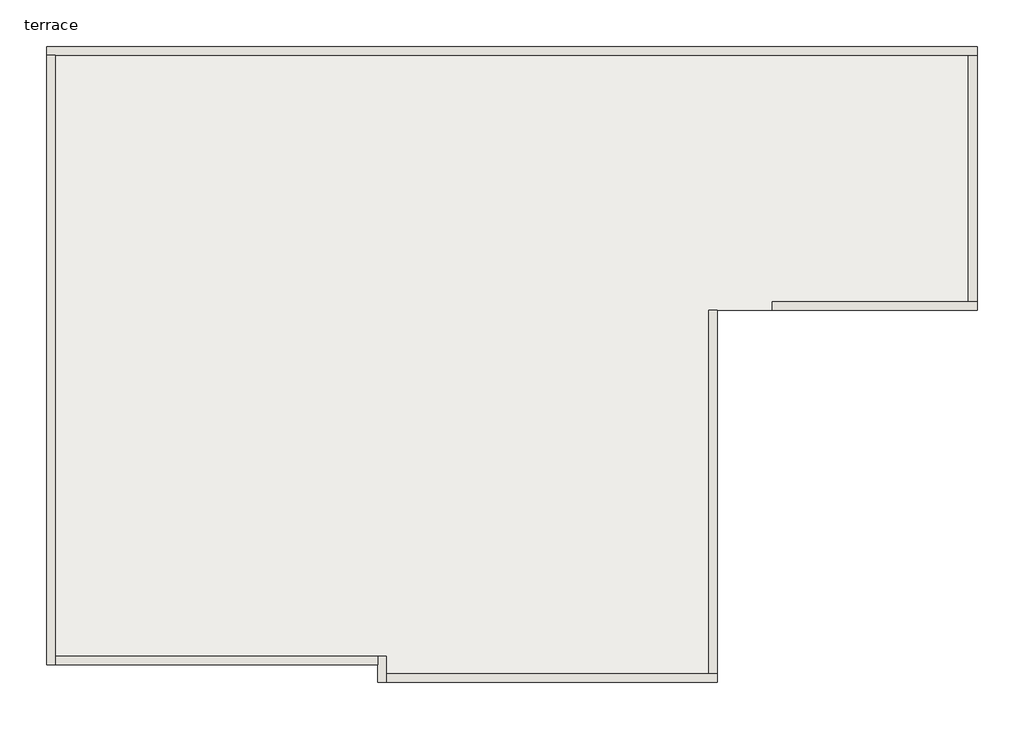
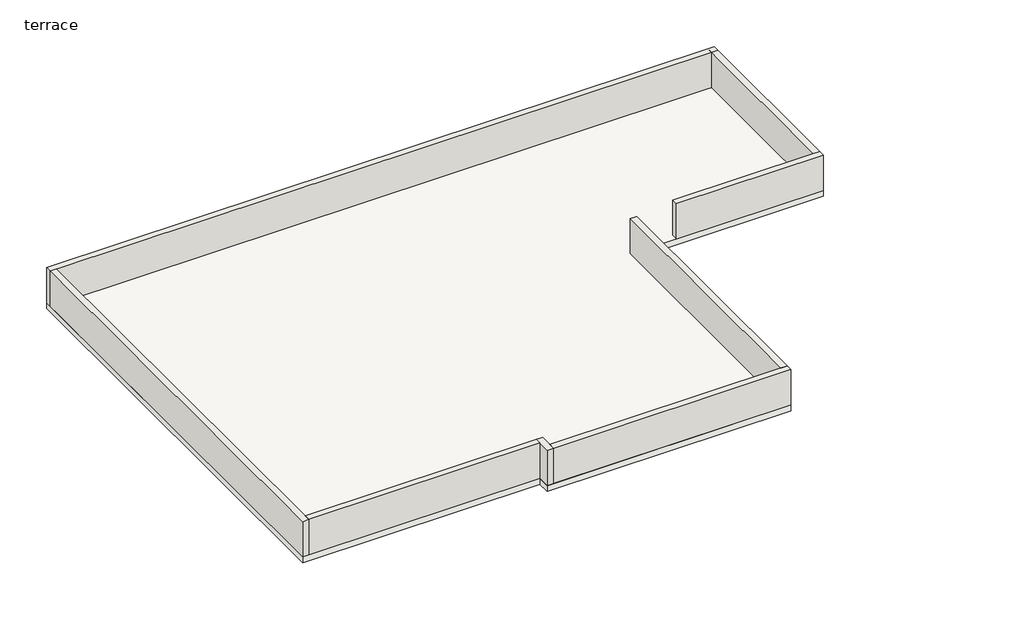
# One storey: 8 walls, 1 slab.
"""IFC4 building model written with IfcOpenShell, lengths in millimetres."""

from ifc_helpers import new_model, si_unit, frame, origin, place, context, project, spatial, polyline, outline, extrude, faceted_brep, element, save

model = new_model("IFC4")

# Units and contexts
model_context = context("Model", 3, world=origin())
ifc_project = project(units=[si_unit("LENGTHUNIT", "METRE", prefix="MILLI")], contexts=[model_context])

# Site, building, storey
site = spatial("IfcSite", under=ifc_project)
building = spatial("IfcBuilding", under=site)
storey = spatial("IfcBuildingStorey", under=building, Name="terrace", Elevation=3810.0)

# Slab
placement = place(None, origin())
element("IfcSlab", 1, ObjectType="Generic - 3", at=placement, inside=storey, context=model_context, shape_type="SweptSolid", body=[
    extrude(outline(polyline([(-2241.5417413, 13089.8965218), (-2241.5417413, 8479.7965218), (-6794.4917413, 8479.7965218), (-6794.4917413, 1964.6965218), (-12738.0917413, 1964.6965218), (-12738.0917413, 2269.4965218), (-18529.2917413, 2269.4965218), (-18529.2917413, 13089.8965218), (-2241.5417413, 13089.8965218)])), frame((0.0, 0.0, 3657.6), z_axis=(0.0, 0.0, 1.0), x_axis=(1.0, 0.0, 0.0)), (0.0, 0.0, 1.0), 152.4),
])

# Walls
element("IfcWall", 2, ObjectType="Generic - 6\"", at=placement, inside=storey, context=model_context, shape_type="Brep", body=[
    faceted_brep([(-5829.2917413, 8473.7492417, 3810.0), (-2247.8917413, 8473.7492417, 3810.0), (-2247.8917413, 8473.7492417, 4724.4), (-5829.2917413, 8473.7492417, 4724.4), (-5829.2917413, 8626.1492417, 3810.0), (-5829.2917413, 8626.1492417, 4724.4), (-2400.2917413, 8626.1492417, 4724.4), (-2247.8917413, 8626.1492417, 4724.4), (-2247.8917413, 8626.1492417, 3810.0), (-2400.2917413, 8626.1492417, 3810.0)], [[[0, 1, 2, 3]], [[4, 5, 6, 7, 8, 9]], [[1, 0, 4, 9, 8]], [[3, 2, 7, 6, 5]], [[0, 3, 5, 4]], [[2, 1, 8, 7]]]),
])
element("IfcWall", 3, ObjectType="Generic - 6\"", at=placement, inside=storey, context=model_context, shape_type="SweptSolid", body=[
    extrude(outline(polyline([(-2247.8917413, 13020.3492417), (-2247.8917413, 8626.1492417), (-2400.2917413, 8626.1492417), (-2400.2917413, 13020.3492417), (-2247.8917413, 13020.3492417)])), frame((0.0, 0.0, 3810.0), z_axis=(0.0, 0.0, 1.0), x_axis=(1.0, 0.0, 0.0)), (0.0, 0.0, 1.0), 914.4),
])
element("IfcWall", 4, ObjectType="Generic - 6\"", at=placement, inside=storey, context=model_context, shape_type="Brep", body=[
    faceted_brep([(-2241.5417413, 13089.8965218, 3810.0), (-18529.2917413, 13089.8965218, 3810.0), (-18529.2917413, 13089.8965218, 4724.4), (-2241.5417413, 13089.8965218, 4724.4), (-2241.5417413, 12937.4965218, 3810.0), (-2241.5417413, 12937.4965218, 4724.4), (-18376.8917413, 12937.4965218, 4724.4), (-18529.2917413, 12937.4965218, 4724.4), (-18529.2917413, 12937.4965218, 3810.0), (-18376.8917413, 12937.4965218, 3810.0)], [[[0, 1, 2, 3]], [[4, 5, 6, 7, 8, 9]], [[1, 0, 4, 9, 8]], [[3, 2, 7, 6, 5]], [[0, 3, 5, 4]], [[2, 1, 8, 7]]]),
])
element("IfcWall", 5, ObjectType="Generic - 6\"", at=placement, inside=storey, context=model_context, shape_type="Brep", body=[
    faceted_brep([(-18529.2917413, 12937.4965218, 3810.0), (-18529.2917413, 2269.4965218, 3810.0), (-18529.2917413, 2269.4965218, 4724.4), (-18529.2917413, 12937.4965218, 4724.4), (-18376.8917413, 12937.4965218, 3810.0), (-18376.8917413, 12937.4965218, 4724.4), (-18376.8917413, 2421.8965218, 4724.4), (-18376.8917413, 2269.4965218, 4724.4), (-18376.8917413, 2269.4965218, 3810.0), (-18376.8917413, 2421.8965218, 3810.0)], [[[0, 1, 2, 3]], [[4, 5, 6, 7, 8, 9]], [[1, 0, 4, 9, 8]], [[3, 2, 7, 6, 5]], [[0, 3, 5, 4]], [[2, 1, 8, 7]]]),
])
element("IfcWall", 6, ObjectType="Generic - 6\"", at=placement, inside=storey, context=model_context, shape_type="SweptSolid", body=[
    extrude(outline(polyline([(-12738.0917413, 2269.4965218), (-18376.8917413, 2269.4965218), (-18376.8917413, 2421.8965218), (-12738.0917413, 2421.8965218), (-12738.0917413, 2269.4965218)])), frame((0.0, 0.0, 3810.0), z_axis=(0.0, 0.0, 1.0), x_axis=(1.0, 0.0, 0.0)), (0.0, 0.0, 1.0), 914.4),
])
element("IfcWall", 7, ObjectType="Generic - 6\"", at=placement, inside=storey, context=model_context, shape_type="Brep", body=[
    faceted_brep([(-12738.0917413, 2421.8965218, 3810.0), (-12738.0917413, 2269.4965218, 3810.0), (-12738.0917413, 1964.6965218, 3810.0), (-12738.0917413, 1964.6965218, 4724.4), (-12738.0917413, 2269.4965218, 4724.4), (-12738.0917413, 2421.8965218, 4724.4), (-12585.6917413, 2421.8965218, 3810.0), (-12585.6917413, 2421.8965218, 4724.4), (-12585.6917413, 2117.0965218, 4724.4), (-12585.6917413, 1964.6965218, 4724.4), (-12585.6917413, 1964.6965218, 3810.0), (-12585.6917413, 2117.0965218, 3810.0)], [[[0, 1, 2, 3, 4, 5]], [[6, 7, 8, 9, 10, 11]], [[2, 1, 0, 6, 11, 10]], [[5, 4, 3, 9, 8, 7]], [[0, 5, 7, 6]], [[3, 2, 10, 9]]]),
])
element("IfcWall", 8, ObjectType="Generic - 6\"", at=placement, inside=storey, context=model_context, shape_type="Brep", body=[
    faceted_brep([(-12585.6917413, 1964.6965218, 3810.0), (-6794.4917413, 1964.6965218, 3810.0), (-6794.4917413, 1964.6965218, 4724.4), (-12585.6917413, 1964.6965218, 4724.4), (-12585.6917413, 2117.0965218, 3810.0), (-12585.6917413, 2117.0965218, 4724.4), (-6946.8917413, 2117.0965218, 4724.4), (-6794.4917413, 2117.0965218, 4724.4), (-6794.4917413, 2117.0965218, 3810.0), (-6946.8917413, 2117.0965218, 3810.0)], [[[0, 1, 2, 3]], [[4, 5, 6, 7, 8, 9]], [[1, 0, 4, 9, 8]], [[3, 2, 7, 6, 5]], [[0, 3, 5, 4]], [[2, 1, 8, 7]]]),
])
element("IfcWall", 9, ObjectType="Generic - 6\"", at=placement, inside=storey, context=model_context, shape_type="SweptSolid", body=[
    extrude(outline(polyline([(-6794.4917413, 8479.7965218), (-6794.4917413, 2117.0965218), (-6946.8917413, 2117.0965218), (-6946.8917413, 8479.7965218), (-6794.4917413, 8479.7965218)])), frame((0.0, 0.0, 3810.0), z_axis=(0.0, 0.0, 1.0), x_axis=(1.0, 0.0, 0.0)), (0.0, 0.0, 1.0), 914.4),
])

save(model, "model.ifc")

# Revit data of these elements
# Type "Generic - 3"
#   Assembly Code = "B1010"
#   Function = 0
#   Layers, outside or top first: 0' - 6" "Concrete, Cast-in-Place gray" (function 1)
# Type "Generic - 6\""
#   Assembly Code = "B2010"
#   Layers, outside or top first: 0' - 6" no material (function 1)
# Element 1 (IfcSlab, "Generic - 3")
#   Height Offset From Level = 0' - 0"
#   Phase Created = New Construction
#   Materials on its faces: "Concrete, Cast-in-Place gray"
# Elements 2, 4, 5, 6, 7, 8, 9 (IfcWall, "Generic - 6\"")
#   Top Offset = 0' - 0"
#   Base Offset = 0' - 0"
#   wall height = 3' - 0"
#   Phase Created = New Construction
#   Base Constraint = terrace
#   Top Constraint = plinth wall
#   Materials on its faces: "3D plant-3", "Default Wall"
# Element 3 (IfcWall, "Generic - 6\"")
#   Top Offset = 0' - 0"
#   Base Offset = 0' - 0"
#   wall height = 3' - 0"
#   Phase Created = New Construction
#   Base Constraint = terrace
#   Top Constraint = plinth wall
#   Materials on its faces: "Default Wall", "3D plant-3"
# Materials
#   "Concrete, Cast-in-Place gray": class "Concrete", colour RGB 192 192 192, transparency 0, Description = "Cast-in-place concrete", Cost = 0
#   "3D plant-3": class "Paint", colour RGB 76 57 38, transparency 0
#   "Default Wall": colour RGB 128 128 128, transparency 0, Cost = 0
